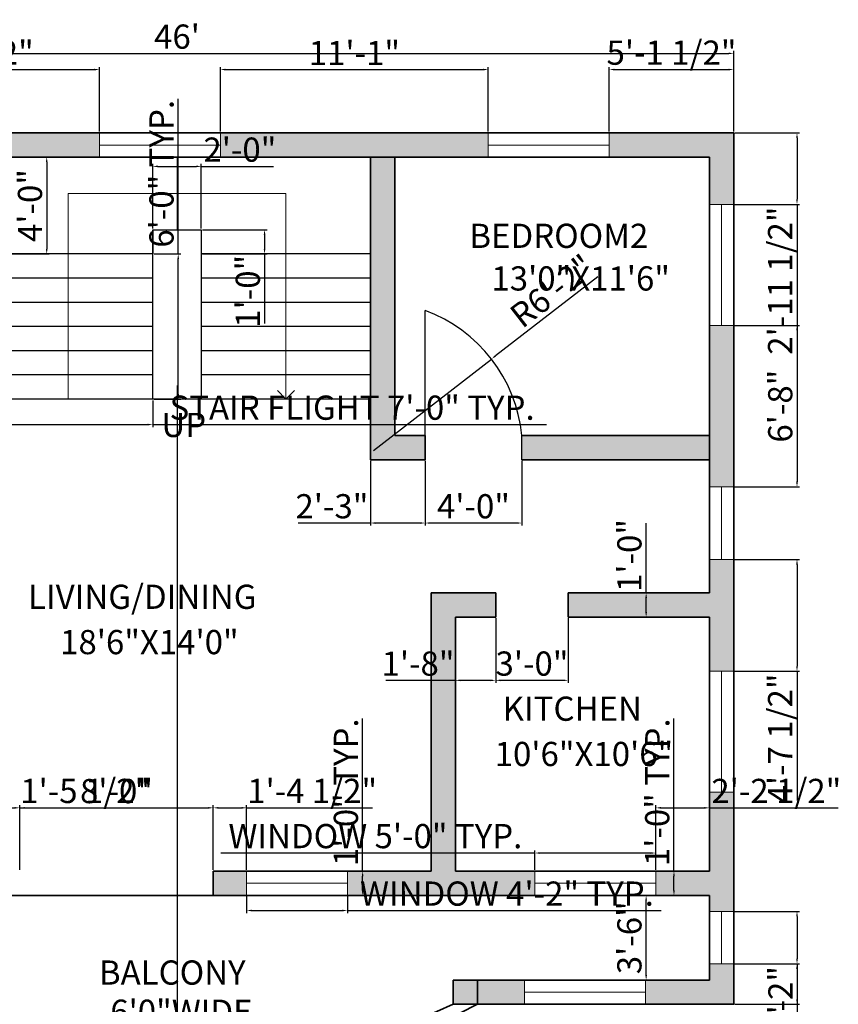
# Model space of a CAD drawing. Units: inches. Extents: x 1749 to 2426, y 1666 to 2412.
# Tile 3 of 3: x 2021 to 2426, y 1924 to 2412. Entities that reach past the tile are written whole.
import ezdxf

# ---------------------------------------------------------------- set-up
doc = ezdxf.new("R2010")
doc.units = ezdxf.units.IN
for name, color, linetype, lineweight in [('A-ANNO-DIMS', 2, 'Continuous', 18), ('A-ANNO-SYMB', 7, 'Continuous', 18), ('A-AREA-IDEN', 4, 'Continuous', 18), ('A-DOOR', 6, 'Continuous', 25), ('A-FLOR-STRS', 7, 'Continuous', 25), ('A-GLAZ', 1, 'Continuous', 18), ('A-WALL', 2, 'Continuous', 35)]:
    doc.layers.add(name, color=color, linetype=linetype, lineweight=lineweight)
doc.layers.add('A-WALL-PATT', color=18, linetype='Continuous', lineweight=13, true_color=0x000000)
doc.styles.get("Standard").update_dxf_attribs({"font": 'arial.ttf'})
doc.dimstyles.new('ISO-25', dxfattribs={"dimtxt": 12, "dimasz": 2.5, "dimexe": 1.25, "dimexo": 0.625, "dimtad": 1, "dimdec": 0, "dimlunit": 3, "dimtxsty": 'Standard', "dimcen": 2.5, "dimadec": 0, "dimazin": 0, "dimtfac": 1, "dimtdec": 0, "dimtmove": 0, "dimatfit": 3, "dimfxl": 1, "dimarcsym": 0})

# ---------------------------------------------------------------- blocks, each defined once
blk = doc.blocks.new('*D1')
at = {"layer": 'A-ANNO-DIMS', "color": 0, "lineweight": -2, "transparency": 16777216}
for p, q in [((1822.59, 2356.85), (1822.59, 2396.9)), ((2374.59, 2356.85), (2374.59, 2396.9)), ((1825.09, 2395.65), (2372.09, 2395.65))]:
    blk.add_line(p, q, dxfattribs=at)
at = {"layer": 'A-ANNO-DIMS', "color": 0, "transparency": 16777216}
for points in [[(1825.09, 2396.07), (1825.09, 2395.23), (1822.59, 2395.65)], [(2372.09, 2396.07), (2372.09, 2395.23), (2374.59, 2395.65)]]:
    blk.add_solid(points, dxfattribs=at)
at = {"layer": 'Defpoints', "color": 0, "transparency": 16777216}
for p in [(2374.59, 2395.65), (1822.59, 2356.22), (2374.59, 2356.22)]:
    blk.add_point(p, dxfattribs=at)
at = {"layer": 'A-ANNO-DIMS', "color": 0, "transparency": 16777216, "insert": (2098.59, 2402.4), "char_height": 12, "attachment_point": 5}
blk.add_mtext("46'", dxfattribs=at)
blk = doc.blocks.new('WIN-60IN')
for p, q in [((12, 60), (0, 60)), ((6, 0), (6, 60)), ((6, 60), (12, 60)), ((0, 0), (12, 0))]:
    blk.add_line(p, q)
blk = doc.blocks.new('WIN-50IN')
for p, q in [((0, 0), (0, 12)), ((50, 12), (50, 0)), ((50, 6), (0, 6)), ((0, 6), (0, 0))]:
    blk.add_line(p, q)
blk = doc.blocks.new('STAIR-FLIGHT-84IN')
for p, q in [((84, 72), (0, 72)), ((84, 60), (0, 60)), ((84, 48), (0, 48)), ((84, 36), (0, 36)), ((84, 24), (0, 24)), ((84, 12), (0, 12)), ((84, 0), (0, 0))]:
    blk.add_line(p, q)
blk = doc.blocks.new('*D7')
at = {"layer": 'A-ANNO-DIMS', "color": 0, "lineweight": -2, "transparency": 16777216}
for p, q in [((2275.99, 1999.22), (2120.39, 1999.22)), ((2275.99, 1990.85), (2275.99, 2000.47)), ((2333.49, 1999.22), (2278.49, 1999.22)), ((2335.99, 1990.85), (2335.99, 2000.47))]:
    blk.add_line(p, q, dxfattribs=at)
at = {"layer": 'A-ANNO-DIMS', "color": 0, "transparency": 16777216}
for points in [[(2278.49, 1999.64), (2278.49, 1998.8), (2275.99, 1999.22)], [(2333.49, 1999.64), (2333.49, 1998.8), (2335.99, 1999.22)]]:
    blk.add_solid(points, dxfattribs=at)
at = {"layer": 'Defpoints', "color": 0, "transparency": 16777216}
for p in [(2275.99, 1999.22), (2275.99, 1990.22), (2335.99, 1990.22)]:
    blk.add_point(p, dxfattribs=at)
at = {"layer": 'A-ANNO-DIMS', "color": 0, "transparency": 16777216, "insert": (2196.94, 2006.05), "char_height": 12, "attachment_point": 5}
blk.add_mtext('WINDOW 5\'-0" TYP.', dxfattribs=at)
blk = doc.blocks.new('*D8')
at = {"layer": 'A-ANNO-DIMS', "color": 0, "lineweight": -2, "transparency": 16777216}
for p, q in [((2344.99, 1990.22), (2344.99, 2065.99)), ((2336.61, 1990.22), (2346.24, 1990.22)), ((2344.99, 1980.72), (2344.99, 1987.72)), ((2336.61, 1978.22), (2346.24, 1978.22))]:
    blk.add_line(p, q, dxfattribs=at)
at = {"layer": 'A-ANNO-DIMS', "color": 0, "transparency": 16777216}
for points in [[(2344.57, 1987.72), (2345.4, 1987.72), (2344.99, 1990.22)], [(2344.57, 1980.72), (2345.4, 1980.72), (2344.99, 1978.22)]]:
    blk.add_solid(points, dxfattribs=at)
at = {"layer": 'Defpoints', "color": 0, "transparency": 16777216}
for p in [(2335.99, 1990.22), (2344.99, 1990.22), (2335.99, 1978.22)]:
    blk.add_point(p, dxfattribs=at)
at = {"layer": 'A-ANNO-DIMS', "color": 0, "transparency": 16777216, "insert": (2338.24, 2029.35), "char_height": 12, "attachment_point": 5, "rotation": 90}
blk.add_mtext('1\'-0" TYP.', dxfattribs=at)
blk = doc.blocks.new('*D11')
at = {"layer": 'A-ANNO-DIMS', "color": 0, "lineweight": -2, "transparency": 16777216}
for p, q in [((2133.12, 1977.6), (2133.12, 1969.47)), ((2183.12, 1977.6), (2183.12, 1969.47)), ((2135.62, 1970.72), (2180.62, 1970.72)), ((2183.12, 1970.72), (2338.72, 1970.72))]:
    blk.add_line(p, q, dxfattribs=at)
at = {"layer": 'A-ANNO-DIMS', "color": 0, "transparency": 16777216}
for points in [[(2135.62, 1971.14), (2135.62, 1970.3), (2133.12, 1970.72)], [(2180.62, 1971.14), (2180.62, 1970.3), (2183.12, 1970.72)]]:
    blk.add_solid(points, dxfattribs=at)
at = {"layer": 'Defpoints', "color": 0, "transparency": 16777216}
for p in [(2133.12, 1978.22), (2183.12, 1978.22), (2183.12, 1970.72)]:
    blk.add_point(p, dxfattribs=at)
at = {"layer": 'A-ANNO-DIMS', "color": 0, "transparency": 16777216, "insert": (2262.17, 1977.55), "char_height": 12, "attachment_point": 5}
blk.add_mtext('WINDOW 4\'-2" TYP.', dxfattribs=at)
blk = doc.blocks.new('*D12')
at = {"layer": 'A-ANNO-DIMS', "color": 0, "lineweight": -2, "transparency": 16777216}
for p, q in [((2190.62, 1990.22), (2190.62, 2065.99)), ((2183.75, 1990.22), (2191.87, 1990.22)), ((2190.62, 1980.72), (2190.62, 1987.72)), ((2183.75, 1978.22), (2191.87, 1978.22))]:
    blk.add_line(p, q, dxfattribs=at)
at = {"layer": 'A-ANNO-DIMS', "color": 0, "transparency": 16777216}
for points in [[(2190.21, 1987.72), (2191.04, 1987.72), (2190.62, 1990.22)], [(2190.21, 1980.72), (2191.04, 1980.72), (2190.62, 1978.22)]]:
    blk.add_solid(points, dxfattribs=at)
at = {"layer": 'Defpoints', "color": 0, "transparency": 16777216}
for p in [(2183.12, 1990.22), (2190.62, 1990.22), (2183.12, 1978.22)]:
    blk.add_point(p, dxfattribs=at)
at = {"layer": 'A-ANNO-DIMS', "color": 0, "transparency": 16777216, "insert": (2183.87, 2029.35), "char_height": 12, "attachment_point": 5, "rotation": 90}
blk.add_mtext('1\'-0" TYP.', dxfattribs=at)
blk = doc.blocks.new('*D13')
at = {"layer": 'A-ANNO-DIMS', "color": 0, "lineweight": -2, "transparency": 16777216}
for p, q in [((2002.59, 2223.6), (2002.59, 2210.37)), ((2086.59, 2223.6), (2086.59, 2210.37)), ((2005.09, 2211.62), (2084.09, 2211.62)), ((2086.59, 2211.62), (2281.72, 2211.62))]:
    blk.add_line(p, q, dxfattribs=at)
at = {"layer": 'A-ANNO-DIMS', "color": 0, "transparency": 16777216}
for points in [[(2005.09, 2212.04), (2005.09, 2211.2), (2002.59, 2211.62)], [(2084.09, 2212.04), (2084.09, 2211.2), (2086.59, 2211.62)]]:
    blk.add_solid(points, dxfattribs=at)
at = {"layer": 'Defpoints', "color": 0, "transparency": 16777216}
for p in [(2002.59, 2224.22), (2086.59, 2224.22), (2086.59, 2211.62)]:
    blk.add_point(p, dxfattribs=at)
at = {"layer": 'A-ANNO-DIMS', "color": 0, "transparency": 16777216, "insert": (2185.41, 2218.45), "char_height": 12, "attachment_point": 5}
blk.add_mtext('STAIR FLIGHT 7\'-0" TYP.', dxfattribs=at)
blk = doc.blocks.new('*D14')
at = {"layer": 'A-ANNO-DIMS', "color": 0, "lineweight": -2, "transparency": 16777216}
for p, q in [((2099.19, 2296.22), (2099.19, 2373.18)), ((2087.22, 2296.22), (2100.44, 2296.22)), ((2099.19, 2226.72), (2099.19, 2293.72)), ((2087.22, 2224.22), (2100.44, 2224.22))]:
    blk.add_line(p, q, dxfattribs=at)
at = {"layer": 'A-ANNO-DIMS', "color": 0, "transparency": 16777216}
for points in [[(2098.77, 2293.72), (2099.61, 2293.72), (2099.19, 2296.22)], [(2098.77, 2226.72), (2099.61, 2226.72), (2099.19, 2224.22)]]:
    blk.add_solid(points, dxfattribs=at)
at = {"layer": 'Defpoints', "color": 0, "transparency": 16777216}
for p in [(2086.59, 2296.22), (2099.19, 2296.22), (2086.59, 2224.22)]:
    blk.add_point(p, dxfattribs=at)
at = {"layer": 'A-ANNO-DIMS', "color": 0, "transparency": 16777216, "insert": (2092.44, 2335.95), "char_height": 12, "attachment_point": 5, "rotation": 90}
blk.add_mtext('6\'-0" TYP.', dxfattribs=at)
blk = doc.blocks.new('*D16')
at = {"layer": 'A-ANNO-DIMS', "color": 0, "lineweight": -2, "transparency": 16777216}
for p, q in [((1921.49, 2356.85), (1921.49, 2388.87)), ((1923.99, 2387.62), (2057.63, 2387.62)), ((2060.13, 2356.85), (2060.13, 2388.87))]:
    blk.add_line(p, q, dxfattribs=at)
at = {"layer": 'A-ANNO-DIMS', "color": 0, "transparency": 16777216}
for points in [[(1923.99, 2388.04), (1923.99, 2387.2), (1921.49, 2387.62)], [(2057.63, 2388.04), (2057.63, 2387.2), (2060.13, 2387.62)]]:
    blk.add_solid(points, dxfattribs=at)
at = {"layer": 'Defpoints', "color": 0, "transparency": 16777216}
for p in [(2060.13, 2387.62), (1921.49, 2356.22), (2060.13, 2356.22)]:
    blk.add_point(p, dxfattribs=at)
at = {"layer": 'A-ANNO-DIMS', "color": 0, "transparency": 16777216, "insert": (1990.81, 2394.45), "char_height": 12, "attachment_point": 5}
blk.add_mtext('11\'-6 1/2"', dxfattribs=at)
blk = doc.blocks.new('*D17')
at = {"layer": 'A-ANNO-DIMS', "color": 0, "lineweight": -2, "transparency": 16777216}
for p, q in [((2120.13, 2356.85), (2120.13, 2388.87)), ((2122.63, 2387.62), (2250.44, 2387.62)), ((2252.94, 2356.85), (2252.94, 2388.87))]:
    blk.add_line(p, q, dxfattribs=at)
at = {"layer": 'A-ANNO-DIMS', "color": 0, "transparency": 16777216}
for points in [[(2122.63, 2388.04), (2122.63, 2387.2), (2120.13, 2387.62)], [(2250.44, 2388.04), (2250.44, 2387.2), (2252.94, 2387.62)]]:
    blk.add_solid(points, dxfattribs=at)
at = {"layer": 'Defpoints', "color": 0, "transparency": 16777216}
for p in [(2252.94, 2387.62), (2120.13, 2356.22), (2252.94, 2356.22)]:
    blk.add_point(p, dxfattribs=at)
at = {"layer": 'A-ANNO-DIMS', "color": 0, "transparency": 16777216, "insert": (2186.54, 2394.27), "char_height": 12, "attachment_point": 5}
blk.add_mtext('11\'-1"', dxfattribs=at)
blk = doc.blocks.new('*D18')
at = {"layer": 'A-ANNO-DIMS', "color": 0, "lineweight": -2, "transparency": 16777216}
for p, q in [((2312.94, 2356.85), (2312.94, 2388.87)), ((2315.44, 2387.62), (2372.09, 2387.62)), ((2374.59, 2356.85), (2374.59, 2388.87))]:
    blk.add_line(p, q, dxfattribs=at)
at = {"layer": 'A-ANNO-DIMS', "color": 0, "transparency": 16777216}
for points in [[(2315.44, 2388.04), (2315.44, 2387.2), (2312.94, 2387.62)], [(2372.09, 2388.04), (2372.09, 2387.2), (2374.59, 2387.62)]]:
    blk.add_solid(points, dxfattribs=at)
at = {"layer": 'Defpoints', "color": 0, "transparency": 16777216}
for p in [(2374.59, 2387.62), (2312.94, 2356.22), (2374.59, 2356.22)]:
    blk.add_point(p, dxfattribs=at)
at = {"layer": 'A-ANNO-DIMS', "color": 0, "transparency": 16777216, "insert": (2343.77, 2394.45), "char_height": 12, "attachment_point": 5}
blk.add_mtext('5\'-1 1/2"', dxfattribs=at)
blk = doc.blocks.new('*D22')
at = {"layer": 'A-ANNO-DIMS', "color": 0, "lineweight": -2, "transparency": 16777216}
for p, q in [((2375.22, 2356.22), (2407.24, 2356.22)), ((2405.99, 2353.72), (2405.99, 2323.3)), ((2375.22, 2320.8), (2407.24, 2320.8)), ((2405.99, 2320.8), (2405.99, 2247.66))]:
    blk.add_line(p, q, dxfattribs=at)
at = {"layer": 'A-ANNO-DIMS', "color": 0, "transparency": 16777216}
for points in [[(2405.57, 2353.72), (2406.41, 2353.72), (2405.99, 2356.22)], [(2405.57, 2323.3), (2406.41, 2323.3), (2405.99, 2320.8)]]:
    blk.add_solid(points, dxfattribs=at)
at = {"layer": 'Defpoints', "color": 0, "transparency": 16777216}
for p in [(2374.59, 2356.22), (2374.59, 2320.8), (2405.99, 2320.8)]:
    blk.add_point(p, dxfattribs=at)
at = {"layer": 'A-ANNO-DIMS', "color": 0, "transparency": 16777216, "insert": (2399.16, 2282.98), "char_height": 12, "attachment_point": 5, "rotation": 90}
blk.add_mtext('2\'-11 1/2"', dxfattribs=at)
blk = doc.blocks.new('*D23')
at = {"layer": 'A-ANNO-DIMS', "color": 0, "lineweight": -2, "transparency": 16777216}
for p, q in [((2375.22, 2260.8), (2407.24, 2260.8)), ((2405.99, 2258.3), (2405.99, 2183.25)), ((2375.22, 2180.75), (2407.24, 2180.75))]:
    blk.add_line(p, q, dxfattribs=at)
at = {"layer": 'A-ANNO-DIMS', "color": 0, "transparency": 16777216}
for points in [[(2405.57, 2258.3), (2406.41, 2258.3), (2405.99, 2260.8)], [(2405.57, 2183.25), (2406.41, 2183.25), (2405.99, 2180.75)]]:
    blk.add_solid(points, dxfattribs=at)
at = {"layer": 'Defpoints', "color": 0, "transparency": 16777216}
for p in [(2374.59, 2260.8), (2374.59, 2180.75), (2405.99, 2180.75)]:
    blk.add_point(p, dxfattribs=at)
at = {"layer": 'A-ANNO-DIMS', "color": 0, "transparency": 16777216, "insert": (2399.24, 2220.77), "char_height": 12, "attachment_point": 5, "rotation": 90}
blk.add_mtext('6\'-8"', dxfattribs=at)
blk = doc.blocks.new('*D24')
at = {"layer": 'A-ANNO-DIMS', "color": 0, "lineweight": -2, "transparency": 16777216}
for p, q in [((2375.22, 2144.75), (2407.24, 2144.75)), ((2405.99, 2142.25), (2405.99, 2091.82)), ((2375.22, 2089.32), (2407.24, 2089.32)), ((2405.99, 2089.32), (2405.99, 2025.23))]:
    blk.add_line(p, q, dxfattribs=at)
at = {"layer": 'A-ANNO-DIMS', "color": 0, "transparency": 16777216}
for points in [[(2405.57, 2142.25), (2406.41, 2142.25), (2405.99, 2144.75)], [(2405.57, 2091.82), (2406.41, 2091.82), (2405.99, 2089.32)]]:
    blk.add_solid(points, dxfattribs=at)
at = {"layer": 'Defpoints', "color": 0, "transparency": 16777216}
for p in [(2374.59, 2144.75), (2374.59, 2089.32), (2405.99, 2089.32)]:
    blk.add_point(p, dxfattribs=at)
at = {"layer": 'A-ANNO-DIMS', "color": 0, "transparency": 16777216, "insert": (2399.16, 2056.02), "char_height": 12, "attachment_point": 5, "rotation": 90}
blk.add_mtext('4\'-7 1/2"', dxfattribs=at)
blk = doc.blocks.new('*D25')
at = {"layer": 'A-ANNO-DIMS', "color": 0, "lineweight": -2, "transparency": 16777216}
for p, q in [((2361.97, 1978.22), (2329.94, 1978.22)), ((2331.19, 1938.72), (2331.19, 1975.72)), ((2361.97, 1936.22), (2329.94, 1936.22))]:
    blk.add_line(p, q, dxfattribs=at)
at = {"layer": 'A-ANNO-DIMS', "color": 0, "transparency": 16777216}
for points in [[(2330.77, 1975.72), (2331.61, 1975.72), (2331.19, 1978.22)], [(2330.77, 1938.72), (2331.61, 1938.72), (2331.19, 1936.22)]]:
    blk.add_solid(points, dxfattribs=at)
at = {"layer": 'Defpoints', "color": 0, "transparency": 16777216}
for p in [(2331.19, 1978.22), (2362.59, 1978.22), (2362.59, 1936.22)]:
    blk.add_point(p, dxfattribs=at)
at = {"layer": 'A-ANNO-DIMS', "color": 0, "transparency": 16777216, "insert": (2324.44, 1957.22), "char_height": 12, "attachment_point": 5, "rotation": 90}
blk.add_mtext('3\'-6"', dxfattribs=at)
blk = doc.blocks.new('*D31')
at = {"layer": 'A-ANNO-DIMS', "color": 0, "lineweight": -2, "transparency": 16777216}
for p, q in [((2221.59, 2193.6), (2221.59, 2161.57)), ((2269.59, 2193.6), (2269.59, 2161.57)), ((2267.09, 2162.82), (2224.09, 2162.82))]:
    blk.add_line(p, q, dxfattribs=at)
at = {"layer": 'A-ANNO-DIMS', "color": 0, "transparency": 16777216}
for points in [[(2224.09, 2163.24), (2224.09, 2162.4), (2221.59, 2162.82)], [(2267.09, 2163.24), (2267.09, 2162.4), (2269.59, 2162.82)]]:
    blk.add_solid(points, dxfattribs=at)
at = {"layer": 'Defpoints', "color": 0, "transparency": 16777216}
for p in [(2221.59, 2194.22), (2269.59, 2194.22), (2221.59, 2162.82)]:
    blk.add_point(p, dxfattribs=at)
at = {"layer": 'A-ANNO-DIMS', "color": 0, "transparency": 16777216, "insert": (2245.59, 2169.57), "char_height": 12, "attachment_point": 5}
blk.add_mtext('4\'-0"', dxfattribs=at)
blk = doc.blocks.new('*D32')
at = {"layer": 'A-ANNO-DIMS', "color": 0, "lineweight": -2, "transparency": 16777216}
for p, q in [((2194.59, 2193.6), (2194.59, 2161.57)), ((2221.59, 2193.6), (2221.59, 2161.57)), ((2194.59, 2162.82), (2158.74, 2162.82)), ((2219.09, 2162.82), (2197.09, 2162.82))]:
    blk.add_line(p, q, dxfattribs=at)
at = {"layer": 'A-ANNO-DIMS', "color": 0, "transparency": 16777216}
for points in [[(2197.09, 2163.24), (2197.09, 2162.4), (2194.59, 2162.82)], [(2219.09, 2163.24), (2219.09, 2162.4), (2221.59, 2162.82)]]:
    blk.add_solid(points, dxfattribs=at)
at = {"layer": 'Defpoints', "color": 0, "transparency": 16777216}
for p in [(2194.59, 2194.22), (2221.59, 2194.22), (2194.59, 2162.82)]:
    blk.add_point(p, dxfattribs=at)
at = {"layer": 'A-ANNO-DIMS', "color": 0, "transparency": 16777216, "insert": (2175.41, 2169.58), "char_height": 12, "attachment_point": 5}
blk.add_mtext('2\'-3"', dxfattribs=at)
blk = doc.blocks.new('*D33')
at = {"layer": 'A-ANNO-DIMS', "color": 0, "lineweight": -2, "transparency": 16777216}
for p, q in [((2003.22, 2344.22), (2035.24, 2344.22)), ((2033.99, 2341.72), (2033.99, 2298.72)), ((2003.22, 2296.22), (2035.24, 2296.22))]:
    blk.add_line(p, q, dxfattribs=at)
at = {"layer": 'A-ANNO-DIMS', "color": 0, "transparency": 16777216}
for points in [[(2033.57, 2341.72), (2034.41, 2341.72), (2033.99, 2344.22)], [(2033.57, 2298.72), (2034.41, 2298.72), (2033.99, 2296.22)]]:
    blk.add_solid(points, dxfattribs=at)
at = {"layer": 'Defpoints', "color": 0, "transparency": 16777216}
for p in [(2002.59, 2344.22), (2002.59, 2296.22), (2033.99, 2296.22)]:
    blk.add_point(p, dxfattribs=at)
at = {"layer": 'A-ANNO-DIMS', "color": 0, "transparency": 16777216, "insert": (2027.24, 2320.22), "char_height": 12, "attachment_point": 5, "rotation": 90}
blk.add_mtext('4\'-0"', dxfattribs=at)
blk = doc.blocks.new('*D34')
at = {"layer": 'A-ANNO-DIMS', "color": 0, "lineweight": -2, "transparency": 16777216}
for p, q in [((2086.59, 2308.85), (2086.59, 2340.87)), ((2089.09, 2339.62), (2108.09, 2339.62)), ((2110.59, 2308.85), (2110.59, 2340.87)), ((2110.59, 2339.62), (2146.45, 2339.62))]:
    blk.add_line(p, q, dxfattribs=at)
at = {"layer": 'A-ANNO-DIMS', "color": 0, "transparency": 16777216}
for points in [[(2089.09, 2340.04), (2089.09, 2339.2), (2086.59, 2339.62)], [(2108.09, 2340.04), (2108.09, 2339.2), (2110.59, 2339.62)]]:
    blk.add_solid(points, dxfattribs=at)
at = {"layer": 'Defpoints', "color": 0, "transparency": 16777216}
for p in [(2110.59, 2339.62), (2086.59, 2308.22), (2110.59, 2308.22)]:
    blk.add_point(p, dxfattribs=at)
at = {"layer": 'A-ANNO-DIMS', "color": 0, "transparency": 16777216, "insert": (2129.77, 2346.37), "char_height": 12, "attachment_point": 5}
blk.add_mtext('2\'-0"', dxfattribs=at)
blk = doc.blocks.new('*D35')
at = {"layer": 'A-ANNO-DIMS', "color": 0, "lineweight": -2, "transparency": 16777216}
for p, q in [((2111.22, 2308.22), (2143.24, 2308.22)), ((2141.99, 2305.72), (2141.99, 2298.72)), ((2111.22, 2296.22), (2143.24, 2296.22)), ((2141.99, 2296.22), (2141.99, 2261.7))]:
    blk.add_line(p, q, dxfattribs=at)
at = {"layer": 'A-ANNO-DIMS', "color": 0, "transparency": 16777216}
for points in [[(2141.57, 2305.72), (2142.41, 2305.72), (2141.99, 2308.22)], [(2141.57, 2298.72), (2142.41, 2298.72), (2141.99, 2296.22)]]:
    blk.add_solid(points, dxfattribs=at)
at = {"layer": 'Defpoints', "color": 0, "transparency": 16777216}
for p in [(2110.59, 2308.22), (2110.59, 2296.22), (2141.99, 2296.22)]:
    blk.add_point(p, dxfattribs=at)
at = {"layer": 'A-ANNO-DIMS', "color": 0, "transparency": 16777216, "insert": (2135.24, 2277.71), "char_height": 12, "attachment_point": 5, "rotation": 90}
blk.add_mtext('1\'-0"', dxfattribs=at)
blk = doc.blocks.new('*D36')
at = {"layer": 'A-ANNO-DIMS', "color": 0, "lineweight": -2, "transparency": 16777216}
for p, q in [((2020.59, 1990.85), (2020.59, 2022.87)), ((2023.09, 2021.62), (2114.09, 2021.62)), ((2116.59, 1990.85), (2116.59, 2022.87))]:
    blk.add_line(p, q, dxfattribs=at)
at = {"layer": 'A-ANNO-DIMS', "color": 0, "transparency": 16777216}
for points in [[(2023.09, 2022.04), (2023.09, 2021.2), (2020.59, 2021.62)], [(2114.09, 2022.04), (2114.09, 2021.2), (2116.59, 2021.62)]]:
    blk.add_solid(points, dxfattribs=at)
at = {"layer": 'Defpoints', "color": 0, "transparency": 16777216}
for p in [(2116.59, 2021.62), (2020.59, 1990.22), (2116.59, 1990.22)]:
    blk.add_point(p, dxfattribs=at)
at = {"layer": 'A-ANNO-DIMS', "color": 0, "transparency": 16777216, "insert": (2068.59, 2028.37), "char_height": 12, "attachment_point": 5}
blk.add_mtext('8\'-0"', dxfattribs=at)
blk = doc.blocks.new('*D37')
at = {"layer": 'A-ANNO-DIMS', "color": 0, "lineweight": -2, "transparency": 16777216}
for p, q in [((2256.59, 2115.6), (2256.59, 2083.57)), ((2292.59, 2115.6), (2292.59, 2083.57)), ((2290.09, 2084.82), (2259.09, 2084.82))]:
    blk.add_line(p, q, dxfattribs=at)
at = {"layer": 'A-ANNO-DIMS', "color": 0, "transparency": 16777216}
for points in [[(2259.09, 2085.24), (2259.09, 2084.4), (2256.59, 2084.82)], [(2290.09, 2085.24), (2290.09, 2084.4), (2292.59, 2084.82)]]:
    blk.add_solid(points, dxfattribs=at)
at = {"layer": 'Defpoints', "color": 0, "transparency": 16777216}
for p in [(2256.59, 2116.22), (2292.59, 2116.22), (2256.59, 2084.82)]:
    blk.add_point(p, dxfattribs=at)
at = {"layer": 'A-ANNO-DIMS', "color": 0, "transparency": 16777216, "insert": (2274.59, 2091.58), "char_height": 12, "attachment_point": 5}
blk.add_mtext('3\'-0"', dxfattribs=at)
blk = doc.blocks.new('*D38')
at = {"layer": 'A-ANNO-DIMS', "color": 0, "lineweight": -2, "transparency": 16777216}
for p, q in [((2236.59, 2115.6), (2236.59, 2083.57)), ((2256.59, 2115.6), (2256.59, 2083.57)), ((2236.59, 2084.82), (2202.07, 2084.82)), ((2254.09, 2084.82), (2239.09, 2084.82))]:
    blk.add_line(p, q, dxfattribs=at)
at = {"layer": 'A-ANNO-DIMS', "color": 0, "transparency": 16777216}
for points in [[(2239.09, 2085.24), (2239.09, 2084.4), (2236.59, 2084.82)], [(2254.09, 2085.24), (2254.09, 2084.4), (2256.59, 2084.82)]]:
    blk.add_solid(points, dxfattribs=at)
at = {"layer": 'Defpoints', "color": 0, "transparency": 16777216}
for p in [(2236.59, 2116.22), (2256.59, 2116.22), (2236.59, 2084.82)]:
    blk.add_point(p, dxfattribs=at)
at = {"layer": 'A-ANNO-DIMS', "color": 0, "transparency": 16777216, "insert": (2218.08, 2091.57), "char_height": 12, "attachment_point": 5}
blk.add_mtext('1\'-8"', dxfattribs=at)
blk = doc.blocks.new('*D39')
at = {"layer": 'A-ANNO-DIMS', "color": 0, "lineweight": -2, "transparency": 16777216}
for p, q in [((2331.19, 2128.22), (2331.19, 2162.74)), ((2361.97, 2128.22), (2329.94, 2128.22)), ((2331.19, 2118.72), (2331.19, 2125.72)), ((2361.97, 2116.22), (2329.94, 2116.22))]:
    blk.add_line(p, q, dxfattribs=at)
at = {"layer": 'A-ANNO-DIMS', "color": 0, "transparency": 16777216}
for points in [[(2330.77, 2125.72), (2331.61, 2125.72), (2331.19, 2128.22)], [(2330.77, 2118.72), (2331.61, 2118.72), (2331.19, 2116.22)]]:
    blk.add_solid(points, dxfattribs=at)
at = {"layer": 'Defpoints', "color": 0, "transparency": 16777216}
for p in [(2331.19, 2128.22), (2362.59, 2128.22), (2362.59, 2116.22)]:
    blk.add_point(p, dxfattribs=at)
at = {"layer": 'A-ANNO-DIMS', "color": 0, "transparency": 16777216, "insert": (2324.44, 2146.73), "char_height": 12, "attachment_point": 5, "rotation": 90}
blk.add_mtext('1\'-0"', dxfattribs=at)
blk = doc.blocks.new('*D42')
at = {"layer": 'A-ANNO-DIMS', "color": 0, "lineweight": -2, "transparency": 16777216}
for p, q in [((2375.22, 1970.3), (2407.24, 1970.3)), ((2405.99, 1967.8), (2405.99, 1946.8)), ((2375.22, 1944.3), (2407.24, 1944.3)), ((2405.99, 1944.3), (2405.99, 1908.45))]:
    blk.add_line(p, q, dxfattribs=at)
at = {"layer": 'A-ANNO-DIMS', "color": 0, "transparency": 16777216}
for points in [[(2405.57, 1967.8), (2406.41, 1967.8), (2405.99, 1970.3)], [(2405.57, 1946.8), (2406.41, 1946.8), (2405.99, 1944.3)]]:
    blk.add_solid(points, dxfattribs=at)
at = {"layer": 'Defpoints', "color": 0, "transparency": 16777216}
for p in [(2374.59, 1970.3), (2374.59, 1944.3), (2405.99, 1944.3)]:
    blk.add_point(p, dxfattribs=at)
at = {"layer": 'A-ANNO-DIMS', "color": 0, "transparency": 16777216, "insert": (2399.34, 1925.13), "char_height": 12, "attachment_point": 5, "rotation": 90}
blk.add_mtext('2\'-2"', dxfattribs=at)
blk = doc.blocks.new('*D43')
at = {"layer": 'A-ANNO-DIMS', "color": 0, "lineweight": -2, "transparency": 16777216}
for p, q in [((2375.22, 1944.3), (2407.24, 1944.3)), ((2405.99, 1941.8), (2405.99, 1926.72)), ((2375.22, 1924.22), (2407.24, 1924.22)), ((2405.99, 1924.22), (2405.99, 1889.7))]:
    blk.add_line(p, q, dxfattribs=at)
at = {"layer": 'A-ANNO-DIMS', "color": 0, "transparency": 16777216}
for points in [[(2405.57, 1941.8), (2406.41, 1941.8), (2405.99, 1944.3)], [(2405.57, 1926.72), (2406.41, 1926.72), (2405.99, 1924.22)]]:
    blk.add_solid(points, dxfattribs=at)
at = {"layer": 'Defpoints', "color": 0, "transparency": 16777216}
for p in [(2374.59, 1944.3), (2374.59, 1924.22), (2405.99, 1924.22)]:
    blk.add_point(p, dxfattribs=at)
at = {"layer": 'A-ANNO-DIMS', "color": 0, "transparency": 16777216, "insert": (2399.24, 1905.71), "char_height": 12, "attachment_point": 5, "rotation": 90}
blk.add_mtext('1\'-8"', dxfattribs=at)
blk = doc.blocks.new('*D49')
at = {"layer": 'A-ANNO-DIMS', "color": 0, "lineweight": -2, "transparency": 16777216}
for p, q in [((2003.29, 1990.85), (2003.29, 2022.87)), ((2005.79, 2021.62), (2018.09, 2021.62)), ((2020.59, 1990.85), (2020.59, 2022.87)), ((2020.59, 2021.62), (2083.07, 2021.62))]:
    blk.add_line(p, q, dxfattribs=at)
at = {"layer": 'A-ANNO-DIMS', "color": 0, "transparency": 16777216}
for points in [[(2005.79, 2022.04), (2005.79, 2021.2), (2003.29, 2021.62)], [(2018.09, 2022.04), (2018.09, 2021.2), (2020.59, 2021.62)]]:
    blk.add_solid(points, dxfattribs=at)
at = {"layer": 'Defpoints', "color": 0, "transparency": 16777216}
for p in [(2020.59, 2021.62), (2003.29, 1990.22), (2020.59, 1990.22)]:
    blk.add_point(p, dxfattribs=at)
at = {"layer": 'A-ANNO-DIMS', "color": 0, "transparency": 16777216, "insert": (2053.08, 2028.45), "char_height": 12, "attachment_point": 5}
blk.add_mtext('1\'-5 1/2"', dxfattribs=at)
blk = doc.blocks.new('*D50')
at = {"layer": 'A-ANNO-DIMS', "color": 0, "lineweight": -2, "transparency": 16777216}
for p, q in [((2116.59, 1990.85), (2116.59, 2022.87)), ((2119.09, 2021.62), (2130.62, 2021.62)), ((2133.12, 1990.85), (2133.12, 2022.87)), ((2133.12, 2021.62), (2195.6, 2021.62))]:
    blk.add_line(p, q, dxfattribs=at)
at = {"layer": 'A-ANNO-DIMS', "color": 0, "transparency": 16777216}
for points in [[(2119.09, 2022.04), (2119.09, 2021.2), (2116.59, 2021.62)], [(2130.62, 2022.04), (2130.62, 2021.2), (2133.12, 2021.62)]]:
    blk.add_solid(points, dxfattribs=at)
at = {"layer": 'Defpoints', "color": 0, "transparency": 16777216}
for p in [(2133.12, 2021.62), (2116.59, 1990.22), (2133.12, 1990.22)]:
    blk.add_point(p, dxfattribs=at)
at = {"layer": 'A-ANNO-DIMS', "color": 0, "transparency": 16777216, "insert": (2165.61, 2028.45), "char_height": 12, "attachment_point": 5}
blk.add_mtext('1\'-4 1/2"', dxfattribs=at)
blk = doc.blocks.new('*D51')
at = {"layer": 'A-ANNO-DIMS', "color": 0, "lineweight": -2, "transparency": 16777216}
for p, q in [((2335.99, 1990.85), (2335.99, 2022.87)), ((2338.49, 2021.62), (2360.09, 2021.62)), ((2362.59, 1990.85), (2362.59, 2022.87)), ((2362.59, 2021.62), (2426.41, 2021.62))]:
    blk.add_line(p, q, dxfattribs=at)
at = {"layer": 'A-ANNO-DIMS', "color": 0, "transparency": 16777216}
for points in [[(2338.49, 2022.04), (2338.49, 2021.2), (2335.99, 2021.62)], [(2360.09, 2022.04), (2360.09, 2021.2), (2362.59, 2021.62)]]:
    blk.add_solid(points, dxfattribs=at)
at = {"layer": 'Defpoints', "color": 0, "transparency": 16777216}
for p in [(2362.59, 2021.62), (2335.99, 1990.22), (2362.59, 1990.22)]:
    blk.add_point(p, dxfattribs=at)
at = {"layer": 'A-ANNO-DIMS', "color": 0, "transparency": 16777216, "insert": (2395.75, 2028.45), "char_height": 12, "attachment_point": 5}
blk.add_mtext('2\'-2 1/2"', dxfattribs=at)
blk = doc.blocks.new('*D56')
at = {"layer": 'A-ANNO-DIMS', "color": 0, "lineweight": -2, "transparency": 16777216}
for p, q in [((2098.59, 2231.02), (2098.59, 1895.02)), ((2098.59, 1666.44), (2098.59, 1892.52))]:
    blk.add_line(p, q, dxfattribs=at)
at = {"layer": 'A-ANNO-DIMS', "color": 0, "transparency": 16777216}
blk.add_solid([(2099.01, 1892.52), (2098.18, 1892.52), (2098.59, 1895.02)], dxfattribs=at)
at = {"layer": 'Defpoints', "color": 0, "transparency": 16777216}
for p in [(2098.59, 2231.02), (2098.59, 1895.02)]:
    blk.add_point(p, dxfattribs=at)
at = {"layer": 'A-ANNO-DIMS', "color": 0, "transparency": 16777216, "insert": (2105.34, 1693.42), "char_height": 12, "attachment_point": 5, "rotation": 270.0001}
blk.add_mtext('R28\'-0"', dxfattribs=at)
blk = doc.blocks.new('*D57')
at = {"layer": 'A-ANNO-DIMS', "color": 0, "lineweight": -2, "transparency": 16777216}
for p, q in [((2098.59, 2211.93), (2098.59, 1887.93)), ((2098.59, 1666.55), (2098.59, 1885.43))]:
    blk.add_line(p, q, dxfattribs=at)
at = {"layer": 'A-ANNO-DIMS', "color": 0, "transparency": 16777216}
blk.add_solid([(2099.01, 1885.43), (2098.18, 1885.43), (2098.59, 1887.93)], dxfattribs=at)
at = {"layer": 'Defpoints', "color": 0, "transparency": 16777216}
for p in [(2098.59, 2211.93), (2098.59, 1887.93)]:
    blk.add_point(p, dxfattribs=at)
at = {"layer": 'A-ANNO-DIMS', "color": 0, "transparency": 16777216, "insert": (2105.34, 1693.53), "char_height": 12, "attachment_point": 5, "rotation": 270.0001}
blk.add_mtext('R27\'-0"', dxfattribs=at)
blk = doc.blocks.new('*D58')
at = {"layer": 'A-ANNO-DIMS', "color": 0, "lineweight": -2, "transparency": 16777216}
for p, q in [((2307.23, 2284.94), (2256.45, 2245.63)), ((2195.96, 2198.8), (2254.48, 2244.1))]:
    blk.add_line(p, q, dxfattribs=at)
at = {"layer": 'A-ANNO-DIMS', "color": 0, "transparency": 16777216}
blk.add_solid([(2256.2, 2245.96), (2256.71, 2245.3), (2254.48, 2244.1)], dxfattribs=at)
at = {"layer": 'Defpoints', "color": 0, "transparency": 16777216}
for p in [(2254.48, 2244.1), (2195.96, 2198.8)]:
    blk.add_point(p, dxfattribs=at)
at = {"layer": 'A-ANNO-DIMS', "color": 0, "transparency": 16777216, "insert": (2285.45, 2276.62), "char_height": 12, "attachment_point": 5, "rotation": 37.7469}
blk.add_mtext('R6\'-2"', dxfattribs=at)

msp = doc.modelspace()

# ---------------------------------------------------------------- hatches: boundary and pattern name
at = {"layer": 'A-WALL-PATT'}
h = msp.add_hatch(color=256, dxfattribs=at)
h.dxf.hatch_style = 1
h.paths.add_polyline_path([(2060.13, 2344.22), (2060.13, 2356.22), (1921.49, 2356.22), (1921.49, 2344.22)])
h = msp.add_hatch(color=256, dxfattribs=at)
h.dxf.hatch_style = 1
h.paths.add_polyline_path([(2120.13, 2356.22), (2120.13, 2344.22), (2252.94, 2344.22), (2252.94, 2356.22)])
h = msp.add_hatch(color=256, dxfattribs=at)
h.dxf.hatch_style = 1
h.paths.add_polyline_path([(2312.94, 2356.22), (2312.94, 2344.22), (2362.59, 2344.22), (2362.59, 2320.8), (2374.59, 2320.8), (2374.59, 2356.22)])
h = msp.add_hatch(color=256, dxfattribs=at)
h.dxf.hatch_style = 1
h.paths.add_polyline_path([(2206.59, 2344.22), (2194.59, 2344.22), (2194.59, 2194.22), (2221.59, 2194.22), (2221.59, 2206.22), (2206.59, 2206.22)])
h = msp.add_hatch(color=256, dxfattribs=at)
h.dxf.hatch_style = 1
h.paths.add_polyline_path([(2374.59, 2260.8), (2362.59, 2260.8), (2362.59, 2180.75), (2374.59, 2180.75)])
h = msp.add_hatch(color=256, dxfattribs=at)
h.dxf.hatch_style = 1
h.paths.add_polyline_path([(2362.59, 2206.22), (2269.59, 2206.22), (2269.59, 2194.22), (2362.59, 2194.22)])
h = msp.add_hatch(color=256, dxfattribs=at)
h.dxf.hatch_style = 1
h.paths.add_polyline_path([(2362.59, 2116.22), (2362.59, 2089.32), (2374.59, 2089.32), (2374.59, 2144.75), (2362.59, 2144.75), (2362.59, 2128.22), (2292.59, 2128.22), (2292.59, 2116.22)])
h = msp.add_hatch(color=256, dxfattribs=at)
h.dxf.hatch_style = 1
h.paths.add_polyline_path([(2236.59, 2116.22), (2256.59, 2116.22), (2256.59, 2128.22), (2224.59, 2128.22), (2224.59, 1990.22), (2183.12, 1990.22), (2183.12, 1978.22), (2275.99, 1978.22), (2275.99, 1990.22), (2236.59, 1990.22)])
h = msp.add_hatch(color=256, dxfattribs=at)
h.dxf.hatch_style = 1
h.paths.add_polyline_path([(2362.59, 1990.22), (2335.99, 1990.22), (2335.99, 1978.22), (2362.59, 1978.22), (2362.59, 1970.3), (2374.59, 1970.3), (2374.59, 2029.32), (2368.59, 2029.32), (2362.59, 2029.32)])
h = msp.add_hatch(color=256, dxfattribs=at)
h.dxf.hatch_style = 1
h.paths.add_polyline_path([(2133.12, 1978.22), (2133.12, 1990.22), (2116.59, 1990.22), (2116.59, 1978.22)])
h = msp.add_hatch(color=256, dxfattribs=at)
h.dxf.hatch_style = 1
h.paths.add_polyline_path([(2362.59, 1936.22), (2330.81, 1936.22), (2330.81, 1924.22), (2374.59, 1924.22), (2374.59, 1944.3), (2362.59, 1944.3)])
h = msp.add_hatch(color=256, dxfattribs=at)
h.dxf.hatch_style = 1
h.paths.add_polyline_path([(2247.59, 1924.22), (2247.59, 1936.22), (2235.59, 1936.22), (2235.59, 1924.22)])
h = msp.add_hatch(color=256, dxfattribs=at)
h.dxf.hatch_style = 1
h.paths.add_polyline_path([(2270.81, 1936.22), (2247.59, 1936.22), (2247.59, 1924.22), (2270.81, 1924.22)])

# ---------------------------------------------------------------- linework, layer by layer
at = {"layer": 'A-ANNO-SYMB'}
for p, q in [((2044.59, 2224.22), (2044.59, 2326.22)), ((2044.59, 2326.22), (2152.59, 2326.22)), ((2152.59, 2326.22), (2152.59, 2224.22)), ((2152.59, 2224.22), (2148.35, 2228.46)), ((2152.59, 2224.22), (2156.83, 2228.46))]:
    msp.add_line(p, q, dxfattribs=at)
at = {"layer": 'A-DOOR'}
for p, q in [((2221.59, 2194.22), (2221.59, 2268.22)), ((2269.59, 2194.22), (2269.59, 2206.22))]:
    msp.add_line(p, q, dxfattribs=at)
msp.add_arc((2195.96, 2198.8), 74, 5.7554, 69.7382, dxfattribs=at)
at = {"layer": 'A-FLOR-STRS'}
for p, q in [((2098.59, 2344.22), (2098.59, 2308.22)), ((2086.59, 2224.22), (2086.59, 2308.22)), ((2086.59, 2308.22), (2098.59, 2308.22)), ((2086.59, 2308.22), (2086.59, 2296.22)), ((2098.59, 2308.22), (2110.59, 2308.22)), ((2110.59, 2308.22), (2110.59, 2224.22)), ((2110.59, 2224.22), (2086.59, 2224.22))]:
    msp.add_line(p, q, dxfattribs=at)
at = {"layer": 'A-GLAZ'}
for p, q in [((2362.59, 2180.75), (2374.59, 2180.75)), ((2368.59, 2180.75), (2368.59, 2144.75)), ((2374.59, 2144.75), (2362.59, 2144.75)), ((2368.59, 2144.75), (2374.59, 2144.75)), ((2362.59, 2089.32), (2374.59, 2089.32)), ((2368.59, 2089.32), (2368.59, 2029.32)), ((2368.59, 2029.32), (2362.59, 2029.32)), ((2368.59, 2029.32), (2374.59, 2029.32)), ((2362.59, 1970.3), (2374.59, 1970.3)), ((2368.59, 1970.3), (2368.59, 1944.3)), ((2374.59, 1944.3), (2362.59, 1944.3)), ((2368.59, 1944.3), (2374.59, 1944.3))]:
    msp.add_line(p, q, dxfattribs=at)
at = {"layer": 'A-WALL'}
for p, q in [((1834.59, 2344.22), (2362.59, 2344.22)), ((2194.59, 2344.22), (2194.59, 2194.22)), ((2206.59, 2344.22), (2206.59, 2206.22)), ((2362.59, 2344.22), (2362.59, 2128.22)), ((2206.59, 2206.22), (2221.59, 2206.22)), ((2221.59, 2206.22), (2221.59, 2194.22)), ((2269.59, 2206.22), (2362.59, 2206.22)), ((2194.59, 2194.22), (2221.59, 2194.22)), ((2269.59, 2194.22), (2362.59, 2194.22)), ((2224.59, 2128.22), (2256.59, 2128.22)), ((2224.59, 2128.22), (2224.59, 1990.22)), ((2256.59, 2128.22), (2256.59, 2116.22)), ((2292.59, 2128.22), (2292.59, 2116.22)), ((2292.59, 2128.22), (2362.59, 2128.22)), ((2236.59, 2116.22), (2256.59, 2116.22)), ((2236.59, 2116.22), (2236.59, 1990.22)), ((2292.59, 2116.22), (2362.59, 2116.22)), ((2362.59, 2116.22), (2362.59, 1990.22)), ((2116.59, 1990.22), (2116.59, 1978.22)), ((2116.59, 1990.22), (2224.59, 1990.22)), ((2236.59, 1990.22), (2362.59, 1990.22)), ((1834.59, 1978.22), (2362.59, 1978.22)), ((2362.59, 1978.22), (2362.59, 1936.22)), ((2362.59, 1936.22), (2235.59, 1936.22)), ((2235.59, 1936.22), (2235.59, 1924.22)), ((2247.59, 1936.22), (2247.59, 1924.22))]:
    msp.add_line(p, q, dxfattribs=at)
msp.add_lwpolyline([(1961.59, 1924.22), (1822.59, 1924.22), (1822.59, 2356.22), (2374.59, 2356.22), (2374.59, 1924.22), (2235.59, 1924.22)], dxfattribs=at)
for centre, radius, start, end in [((2098.59, 2211.93), 324, 242.6209, 297.3791), ((2098.59, 2231.02), 336, 245.9372, 294.0628)]:
    msp.add_arc(centre, radius, start, end, dxfattribs=at)

# ---------------------------------------------------------------- block references
at = {"layer": 'A-FLOR-STRS'}
for p in [(2002.59, 2224.22), (2110.59, 2224.22)]:
    msp.add_blockref('STAIR-FLIGHT-84IN', p, dxfattribs=at)
at = {"layer": 'A-GLAZ', "extrusion": (0, 0, -1), "zscale": -1}
for p, rotation in [((-2060.13, 2344.22), 89.99999999999896), ((-2252.94, 2344.22), 89.99999999999896), ((-2330.81, 1936.22), 270.0000000000003)]:
    msp.add_blockref('WIN-60IN', p, dxfattribs=dict(at, rotation=rotation))
at = {"layer": 'A-GLAZ'}
for p, rotation in [((2374.59, 2320.8), 180), ((2335.99, 1978.22), 90)]:
    msp.add_blockref('WIN-60IN', p, dxfattribs=dict(at, rotation=rotation))
msp.add_blockref('WIN-50IN', (2133.12, 1978.22), dxfattribs=at)

# ---------------------------------------------------------------- texts
at = {"layer": 'A-ANNO-SYMB'}
msp.add_attdef('UP', (2090.87, 2205.43), '', height=12, dxfattribs=at)
at = {"layer": 'A-AREA-IDEN'}
for tag, p in [('BEDROOM2', (2243.54, 2299.2)), ('13\'0"X11\'6"', (2254.48, 2278.07)), ('LIVING/DINING', (2024.77, 2120.25)), ('18\'6"X14\'0"', (2040.64, 2097.79)), ('KITCHEN', (2260.06, 2064.78)), ('10\'6"X10\'6"', (2256.1, 2042.32)), ('BALCONY', (2059.89, 1933.97)), ('6\'0"WIDE', (2065.51, 1914.54))]:
    msp.add_attdef(tag, p, '', height=12, dxfattribs=at)

# ---------------------------------------------------------------- dimensions: what is measured, and where the dimension line sits
at = {"layer": 'A-ANNO-DIMS'}
for base, p1, p2, override, picture, middle in [((2060.13, 2387.62), (1921.49, 2356.22), (2060.13, 2356.22), {"dimdec": 1, "dimlfac": 1, "dimrnd": 0, "dimzin": 1, "dimdsep": 46, "dimlunit": 4, "dimfrac": 2}, '*D16', (1990.81, 2394.45)), ((2374.5915, 2387.6209), (2312.94, 2356.2209), (2374.5915, 2356.2209), {"dimdec": 1, "dimlfac": 1, "dimrnd": 0, "dimzin": 1, "dimdsep": 46, "dimlunit": 4, "dimfrac": 2}, '*D18', (2343.7658, 2394.4506)), ((2374.59, 2395.65), (1822.59, 2356.22), (2374.59, 2356.22), {"dimclrd": 0, "dimclre": 0, "dimclrt": 0}, '*D1', (2098.59, 2402.4)), ((2252.94, 2387.62), (2120.13, 2356.22), (2252.94, 2356.22), {"dimdec": 1, "dimlfac": 1, "dimrnd": 0, "dimzin": 1, "dimdsep": 46, "dimlunit": 4, "dimfrac": 2}, '*D17', (2186.54, 2394.27)), ((2110.59, 2339.62), (2086.59, 2308.22), (2110.59, 2308.22), {"dimdec": 1, "dimlfac": 1, "dimrnd": 0, "dimzin": 1, "dimdsep": 46, "dimlunit": 4, "dimfrac": 2}, '*D34', (2129.77, 2346.37)), ((2133.12, 2021.62), (2116.59, 1990.22), (2133.12, 1990.22), {"dimdec": 1, "dimlfac": 1, "dimrnd": 0, "dimzin": 1, "dimdsep": 46, "dimlunit": 4, "dimfrac": 2}, '*D50', (2165.61, 2028.45)), ((2362.59, 2021.62), (2335.99, 1990.22), (2362.59, 1990.22), {"dimdec": 1, "dimlfac": 1, "dimrnd": 0, "dimzin": 1, "dimdsep": 46, "dimlunit": 4, "dimfrac": 2}, '*D51', (2395.75, 2028.45)), ((2116.59, 2021.62), (2020.59, 1990.22), (2116.59, 1990.22), {"dimdec": 1, "dimlfac": 1, "dimrnd": 0, "dimzin": 1, "dimdsep": 46, "dimlunit": 4, "dimfrac": 2}, '*D36', (2068.59, 2028.37))]:
    dim = msp.add_linear_dim(base=base, p1=p1, p2=p2, dimstyle='ISO-25', override=override, dxfattribs=at)
    dim.commit()
    dim.dimension.update_dxf_attribs({"geometry": picture, "text_midpoint": middle})
for base, p1, p2, angle, text, picture, middle in [((2099.19, 2296.22), (2086.59, 2224.22), (2086.59, 2296.22), 90, '<> TYP.', '*D14', (2092.44, 2335.95)), ((2190.62, 1990.22), (2183.12, 1978.22), (2183.12, 1990.22), 90, '<> TYP.', '*D12', (2183.87, 2029.35)), ((2344.99, 1990.22), (2335.99, 1978.22), (2335.99, 1990.22), 90, '<> TYP.', '*D8', (2338.24, 2029.35)), ((2275.99, 1999.22), (2335.99, 1990.22), (2275.99, 1990.22), 180, 'WINDOW <> TYP.', '*D7', (2196.94, 2006.05))]:
    dim = msp.add_linear_dim(base=base, p1=p1, p2=p2, angle=angle, text=text, dimstyle='ISO-25', override={"dimdec": 1, "dimlfac": 1, "dimrnd": 0, "dimzin": 1, "dimdsep": 46, "dimlunit": 4, "dimfrac": 2}, dxfattribs=at)
    dim.commit()
    dim.dimension.update_dxf_attribs({"geometry": picture, "text_midpoint": middle})
for base, p1, p2, angle, picture, middle in [((2405.99, 2320.8), (2374.59, 2356.22), (2374.59, 2320.8), 90, '*D22', (2399.16, 2282.98)), ((2033.99, 2296.22), (2002.59, 2344.22), (2002.59, 2296.22), 270, '*D33', (2027.24, 2320.22)), ((2141.99, 2296.22), (2110.59, 2308.22), (2110.59, 2296.22), 270, '*D35', (2135.24, 2277.71)), ((2405.9915, 2180.7457), (2374.5915, 2260.7963), (2374.5915, 2180.7457), 90, '*D23', (2399.2396, 2220.771)), ((2194.59, 2162.82), (2221.59, 2194.22), (2194.59, 2194.22), 180, '*D32', (2175.41, 2169.58)), ((2221.59, 2162.82), (2269.59, 2194.22), (2221.59, 2194.22), 180, '*D31', (2245.59, 2169.57)), ((2331.19, 2128.22), (2362.59, 2116.22), (2362.59, 2128.22), 90, '*D39', (2324.44, 2146.73)), ((2405.99, 2089.32), (2374.59, 2144.75), (2374.59, 2089.32), 90, '*D24', (2399.16, 2056.02)), ((2236.59, 2084.82), (2256.59, 2116.22), (2236.59, 2116.22), 180, '*D38', (2218.08, 2091.57)), ((2256.59, 2084.82), (2292.59, 2116.22), (2256.59, 2116.22), 180, '*D37', (2274.59, 2091.58)), ((2020.59, 2021.62), (2003.29, 1990.22), (2020.59, 1990.22), 0, '*D49', (2053.08, 2028.45)), ((2331.19, 1978.22), (2362.59, 1936.22), (2362.59, 1978.22), 90, '*D25', (2324.44, 1957.22)), ((2405.99, 1944.3), (2374.59, 1970.3), (2374.59, 1944.3), 270, '*D42', (2399.34, 1925.13)), ((2405.99, 1924.22), (2374.59, 1944.3), (2374.59, 1924.22), 270, '*D43', (2399.24, 1905.71))]:
    dim = msp.add_linear_dim(base=base, p1=p1, p2=p2, angle=angle, dimstyle='ISO-25', override={"dimdec": 1, "dimlfac": 1, "dimrnd": 0, "dimzin": 1, "dimdsep": 46, "dimlunit": 4, "dimfrac": 2}, dxfattribs=at)
    dim.commit()
    dim.dimension.update_dxf_attribs({"geometry": picture, "text_midpoint": middle})
for center, mpoint, picture, middle in [((2195.96, 2198.8), (2254.48, 2244.1), '*D58', (2289.59, 2271.28)), ((2098.59, 2231.02), (2098.59, 1895.02), '*D56', (2098.59, 1693.42)), ((2098.59, 2211.93), (2098.59, 1887.93), '*D57', (2098.59, 1693.53))]:
    dim = msp.add_radius_dim(center=center, mpoint=mpoint, dimstyle='ISO-25', override={"dimdec": 1, "dimlfac": 1, "dimrnd": 0, "dimzin": 1, "dimdsep": 46, "dimlunit": 4, "dimfrac": 2}, dxfattribs=at)
    dim.commit()
    dim.dimension.update_dxf_attribs({"geometry": picture, "text_midpoint": middle, "dimtype": 164})
for base, p1, p2, text, picture, middle in [((2086.59, 2211.62), (2002.59, 2224.22), (2086.59, 2224.22), 'STAIR FLIGHT <> TYP.', '*D13', (2185.41, 2218.45)), ((2183.12, 1970.72), (2133.12, 1978.22), (2183.12, 1978.22), 'WINDOW <> TYP.', '*D11', (2262.17, 1977.55))]:
    dim = msp.add_linear_dim(base=base, p1=p1, p2=p2, text=text, dimstyle='ISO-25', override={"dimdec": 1, "dimlfac": 1, "dimrnd": 0, "dimzin": 1, "dimdsep": 46, "dimlunit": 4, "dimfrac": 2}, dxfattribs=at)
    dim.commit()
    dim.dimension.update_dxf_attribs({"geometry": picture, "text_midpoint": middle})

doc.saveas('drawing.dxf')
